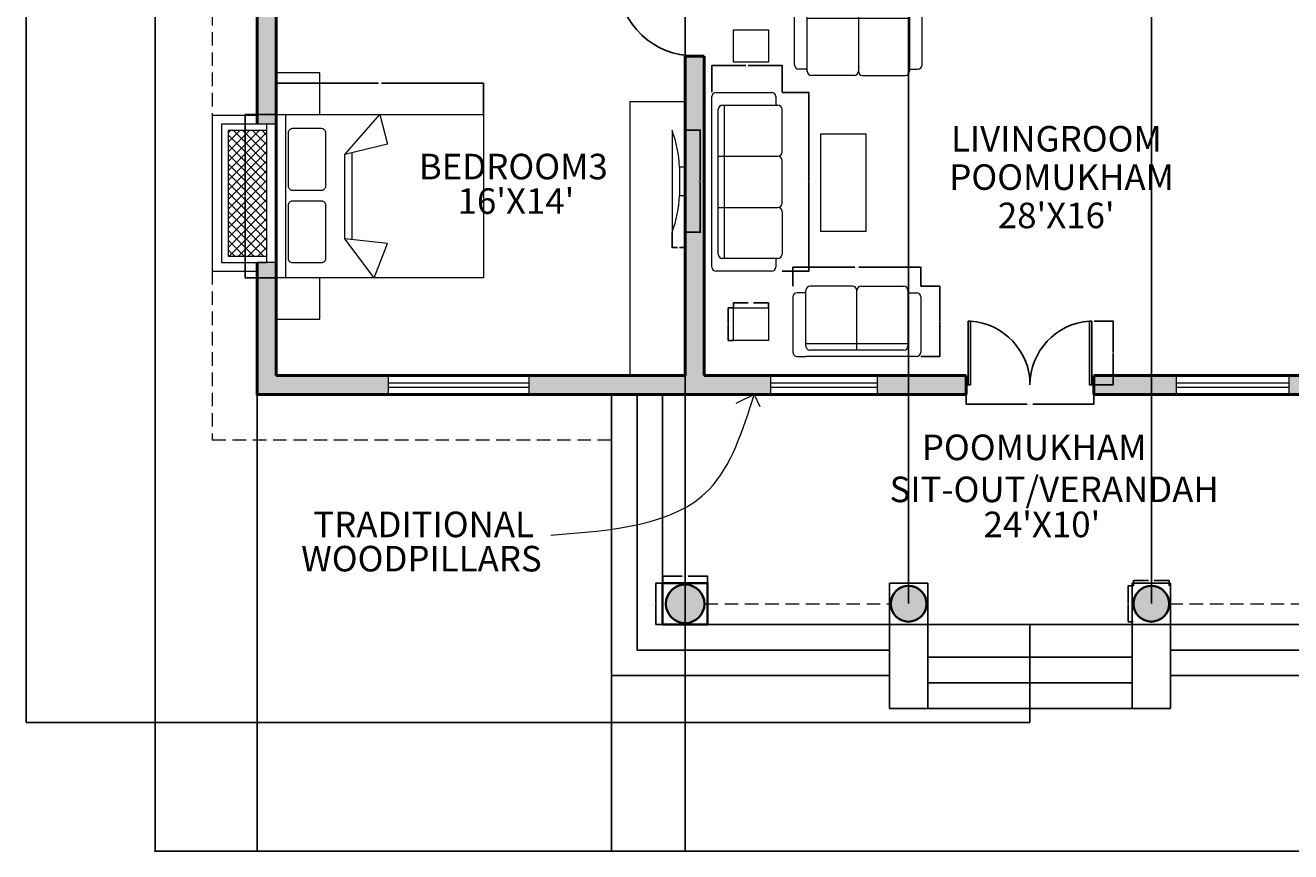
# Model space of a CAD drawing. Units: inches. Extents: x 2743 to 3669, y 1014 to 2282.
# Tile 1 of 5: x 2743 to 3337, y 1014 to 1403. Entities that reach past the tile are written whole.
import ezdxf

# ---------------------------------------------------------------- set-up
doc = ezdxf.new("R2010")
doc.units = ezdxf.units.IN
doc.linetypes.add('DASHED2', pattern=[9.525, 6.35, -3.175])
for name, color, linetype, lineweight in [('A-ANNO-DIMS', 2, 'Continuous', 18), ('A-ANNO-SYMB', 7, 'Continuous', 18), ('A-ANNO-TEXT', 4, 'Continuous', 18), ('A-AREA-IDEN', 4, 'Continuous', 18), ('A-COLS', 7, 'Continuous', 35), ('A-DOOR', 211, 'Continuous', 25), ('A-EQPM', 51, 'Continuous', 18), ('A-FLOR-CASE', 51, 'Continuous', 18), ('A-FLOR-STRS', 7, 'Continuous', 25), ('A-FURN', 111, 'Continuous', 18), ('A-GLAZ', 40, 'Continuous', 20), ('A-GLAZ-PATT', 8, 'Continuous', 13), ('A-ROOF', 7, 'Continuous', 20), ('A-ROOF-OVHD', 8, 'DASHED2', 18), ('A-WALL', 7, 'Continuous', 50)]:
    doc.layers.add(name, color=color, linetype=linetype, lineweight=lineweight)
doc.layers.add('A-COLS-PATT', color=47, linetype='Continuous', lineweight=13, true_color=0x726c55)
doc.layers.add('A-WALL-PATT', color=47, linetype='Continuous', lineweight=13, true_color=0x726c55)
doc.styles.get("Standard").update_dxf_attribs({"font": 'arial.ttf'})
doc.dimstyles.get("Standard").update_dxf_attribs({"dimtxt": 0.18, "dimasz": 0.18, "dimexe": 0.18, "dimexo": 0.0625, "dimgap": 0.09, "dimtad": 0, "dimtih": 1, "dimtoh": 1, "dimdec": 4, "dimzin": 0, "dimdsep": 46, "dimtxsty": 'Standard', "dimcen": 0.09, "dimadec": 0, "dimazin": 0, "dimtfac": 1, "dimtdec": 4, "dimtofl": 0, "dimtmove": 0, "dimatfit": 3, "dimfxl": 1, "dimtolj": 1, "dimtzin": 0, "dimarcsym": 0})

# ---------------------------------------------------------------- blocks, each defined once
blk = doc.blocks.new('DOOR-PAIR-60IN')
for p, q in [((0, 30), (1, 30)), ((1, 30), (1, 0)), ((2, 30), (1, 30)), ((2, 0), (2, 30)), ((58, 0), (58, 30)), ((58, 30), (59, 30)), ((60, 30), (59, 30)), ((59, 30), (59, 0)), ((1, 0), (2, 0)), ((59, 0), (58, 0))]:
    blk.add_line(p, q)
for centre, start, end in [((0, 29.93), 273.82241, 0.12746), ((60, 29.93), 179.99998, 266.1773)]:
    blk.add_arc(centre, 30, start, end)
blk = doc.blocks.new('DOOR-SINGLE-36IN')
for p, q in [((1, 0), (1, 36)), ((1, 36), (2, 36)), ((2, 36), (2, 0)), ((0, 0), (1, 0)), ((2, 0), (1, 0))]:
    blk.add_line(p, q)
blk.add_arc((0, 0.06), 36, 359.91152, 86.81533)
blk = doc.blocks.new('BED-DOUBLE')
for p, q in [((4.31, 76.75), (4.31, 0)), ((32.31, 57.96), (48.69, 76.75)), ((48.69, 76.75), (52.23, 62.72)), ((52.23, 62.72), (32.31, 57.96)), ((32.31, 18.34), (32.31, 57.96)), ((35.7, 17.95), (35.72, 58.78)), ((46.06, 0), (32.31, 18.34)), ((52.23, 16.05), (32.31, 18.34)), ((46.06, 0), (52.23, 16.05))]:
    blk.add_line(p, q)
blk.add_lwpolyline([(0, 76.75), (97.38, 76.75), (97.38, 0), (0, 0)], close=True)
for points in [[(7.76, 70.21), (21.16, 70.21, -0.414214), (23.16, 68.21), (23.16, 43, -0.414214), (21.16, 41), (7.76, 41, -0.414214), (5.76, 43), (5.76, 68.21, -0.414214)], [(7.76, 36.18), (21.16, 36.18, -0.414214), (23.16, 34.18), (23.16, 8.97, -0.414214), (21.16, 6.97), (7.76, 6.97, -0.414214), (5.76, 8.97), (5.76, 34.18, -0.414214)]]:
    blk.add_lwpolyline(points, format="xyb", close=True)
blk = doc.blocks.new('NIGHTSTAND')
blk.add_lwpolyline([(0, 0), (20.5, 0), (20.5, 19.45), (0, 19.45)], close=True)
blk = doc.blocks.new('TABLE-END')
blk.add_lwpolyline([(0, 15.26), (16.38, 15.26), (16.38, 0), (0, 0)], close=True)
blk = doc.blocks.new('SOFA-TWO-SEAT')
for p, q in [((5, 60), (31, 60)), ((2, 54), (28, 54)), ((3, 54), (3, 58)), ((27, 54), (27, 6)), ((33, 58), (33, 6)), ((0, 32), (0, 52)), ((30, 52), (30, 8)), ((30, 30), (2, 30)), ((2, 30), (2, 30)), ((0, 28), (0, 8)), ((28, 6), (2, 6)), ((2, 6), (2, 6)), ((3, 6), (3, 2)), ((33, 2), (33, 6)), ((5, 0), (31, 0))]:
    blk.add_line(p, q)
for centre, start, end in [((5, 58), 90, 180), ((31, 58), 0, 90), ((2, 52), 90, 180), ((28, 52), 0, 90), ((2, 32), 180, 270), ((2, 28), 90, 180), ((2, 8), 180, 270), ((28, 8), 270, 0), ((5, 2), 180, 270), ((31, 2), 270, 0)]:
    blk.add_arc(centre, 2, start, end)
blk = doc.blocks.new('SOFA-THREE-SEAT')
for p, q in [((0, 5), (0, 31)), ((2, 33), (82, 33)), ((8, 30), (76, 30)), ((30, 30), (30, 2)), ((54, 30), (54, 2)), ((84, 31), (84, 5)), ((6, 2), (6, 28)), ((6, 27), (78, 27)), ((78, 28), (78, 2)), ((6, 3), (2, 3)), ((30, 2), (30, 2)), ((54, 2), (54, 2)), ((82, 3), (78, 3)), ((28, 0), (8, 0)), ((32, 0), (52, 0)), ((56, 0), (76, 0))]:
    blk.add_line(p, q)
for centre, start, end in [((2, 31), 90, 180), ((8, 28), 90, 180), ((76, 28), 0, 90), ((82, 31), 0, 90), ((2, 5), 180, 270), ((8, 2), 180, 270), ((28, 2), 270, 0), ((32, 2), 180, 270), ((52, 2), 270, 0), ((56, 2), 180, 270), ((76, 2), 270, 0), ((82, 5), 270, 0)]:
    blk.add_arc(centre, 2, start, end)
blk = doc.blocks.new('TV-SCREEN')
for p, q in [((6.11, 0), (6.11, 47.89)), ((2.64, 30.63), (0, 30.63)), ((2.64, 17.25), (2.64, 30.63)), ((0, 17.25), (2.64, 17.25))]:
    blk.add_line(p, q)
for centre, radius, start, end in [((54.67, 29.14), 52.05, 158.88993, 178.35791), ((54.74, 18.76), 52.13, 181.66464, 201.09645)]:
    blk.add_arc(centre, radius, start, end)
blk = doc.blocks.new('POST-SITOUT-OUTER')
blk.add_lwpolyline([(0, 0), (21.09, 0), (21.09, 19.48), (0, 19.48)], close=True)
blk.add_circle((10.55, 9.74), 9.06)
blk = doc.blocks.new('POST-SITOUT-INNER')
blk.add_circle((8.4, 8.4), 8.4)
blk = doc.blocks.new('*D30')
at = {"layer": 'A-ANNO-DIMS', "color": 0, "lineweight": -2, "transparency": 16777216}
for p, q in [((2860.8, 1360.75), (2860.8, 1375.47)), ((2860.98, 1375.29), (2908.67, 1375.29)), ((2958, 1375.29), (2910.31, 1375.29)), ((2958.18, 1360.75), (2958.18, 1375.47))]:
    blk.add_line(p, q, dxfattribs=at)
at = {"layer": 'A-ANNO-DIMS', "color": 0, "transparency": 16777216}
for points in [[(2860.98, 1375.32), (2860.98, 1375.26), (2860.8, 1375.29)], [(2958, 1375.32), (2958, 1375.26), (2958.18, 1375.29)]]:
    blk.add_solid(points, dxfattribs=at)
at = {"layer": 'Defpoints', "color": 0, "transparency": 16777216}
for p in [(2958.18, 1375.29), (2860.8, 1360.68), (2958.18, 1360.68)]:
    blk.add_point(p, dxfattribs=at)
at = {"layer": 'A-ANNO-DIMS', "color": 0, "transparency": 16777216, "insert": (2909.49, 1375.29), "char_height": 0.18, "attachment_point": 5}
blk.add_mtext('\\A1;BED 97 TYP.', dxfattribs=at)
blk = doc.blocks.new('*D31')
at = {"layer": 'A-ANNO-DIMS', "color": 0, "lineweight": -2, "transparency": 16777216}
for p, q in [((2860.73, 1360.68), (2846.01, 1360.68)), ((2846.19, 1360.5), (2846.19, 1322.49)), ((2846.19, 1284.12), (2846.19, 1322.13)), ((2860.73, 1283.94), (2846.01, 1283.94))]:
    blk.add_line(p, q, dxfattribs=at)
at = {"layer": 'A-ANNO-DIMS', "color": 0, "transparency": 16777216}
for points in [[(2846.16, 1360.5), (2846.22, 1360.5), (2846.19, 1360.68)], [(2846.16, 1284.12), (2846.22, 1284.12), (2846.19, 1283.94)]]:
    blk.add_solid(points, dxfattribs=at)
at = {"layer": 'Defpoints', "color": 0, "transparency": 16777216}
for p in [(2846.19, 1360.68), (2860.8, 1360.68), (2860.8, 1283.94)]:
    blk.add_point(p, dxfattribs=at)
at = {"layer": 'A-ANNO-DIMS', "color": 0, "transparency": 16777216, "insert": (2846.19, 1322.31), "char_height": 0.18, "attachment_point": 5}
blk.add_mtext('\\A1;77 TYP.', dxfattribs=at)
blk = doc.blocks.new('*D32')
at = {"layer": 'A-ANNO-DIMS', "color": 0, "lineweight": -2, "transparency": 16777216}
for p, q in [((3184.8, 1233.53), (3184.8, 1224.41)), ((3244.8, 1233.53), (3244.8, 1224.41)), ((3184.98, 1224.59), (3213.53, 1224.59)), ((3244.62, 1224.59), (3216.06, 1224.59))]:
    blk.add_line(p, q, dxfattribs=at)
at = {"layer": 'A-ANNO-DIMS', "color": 0, "transparency": 16777216}
for points in [[(3184.98, 1224.62), (3184.98, 1224.56), (3184.8, 1224.59)], [(3244.62, 1224.62), (3244.62, 1224.56), (3244.8, 1224.59)]]:
    blk.add_solid(points, dxfattribs=at)
at = {"layer": 'Defpoints', "color": 0, "transparency": 16777216}
for p in [(3184.8, 1233.59), (3244.8, 1233.59), (3184.8, 1224.59)]:
    blk.add_point(p, dxfattribs=at)
at = {"layer": 'A-ANNO-DIMS', "color": 0, "transparency": 16777216, "insert": (3214.8, 1224.59), "char_height": 0.18, "attachment_point": 5}
blk.add_mtext('\\A1;DOOR PAIR 60 TYP.', dxfattribs=at)
blk = doc.blocks.new('*D33')
at = {"layer": 'A-ANNO-DIMS', "color": 0, "lineweight": -2, "transparency": 16777216}
for p, q in [((3244.86, 1263.59), (3253.98, 1263.59)), ((3253.8, 1263.41), (3253.8, 1248.78)), ((3253.8, 1233.77), (3253.8, 1248.41)), ((3244.86, 1233.59), (3253.98, 1233.59))]:
    blk.add_line(p, q, dxfattribs=at)
at = {"layer": 'A-ANNO-DIMS', "color": 0, "transparency": 16777216}
for points in [[(3253.83, 1263.41), (3253.77, 1263.41), (3253.8, 1263.59)], [(3253.83, 1233.77), (3253.77, 1233.77), (3253.8, 1233.59)]]:
    blk.add_solid(points, dxfattribs=at)
at = {"layer": 'Defpoints', "color": 0, "transparency": 16777216}
for p in [(3244.8, 1263.59), (3244.8, 1233.59), (3253.8, 1233.59)]:
    blk.add_point(p, dxfattribs=at)
at = {"layer": 'A-ANNO-DIMS', "color": 0, "transparency": 16777216, "insert": (3253.8, 1248.59), "char_height": 0.18, "attachment_point": 5}
blk.add_mtext('\\A1;30 TYP.', dxfattribs=at)
blk = doc.blocks.new('*D38')
at = {"layer": 'A-ANNO-DIMS', "color": 0, "lineweight": -2, "transparency": 16777216}
for p, q in [((3103.49, 1280.01), (3103.49, 1289.12)), ((3103.67, 1288.94), (3132.59, 1288.94)), ((3163.31, 1288.94), (3134.4, 1288.94)), ((3163.49, 1280.01), (3163.49, 1289.12))]:
    blk.add_line(p, q, dxfattribs=at)
at = {"layer": 'A-ANNO-DIMS', "color": 0, "transparency": 16777216}
for points in [[(3103.67, 1288.97), (3103.67, 1288.91), (3103.49, 1288.94)], [(3163.31, 1288.97), (3163.31, 1288.91), (3163.49, 1288.94)]]:
    blk.add_solid(points, dxfattribs=at)
at = {"layer": 'Defpoints', "color": 0, "transparency": 16777216}
for p in [(3163.49, 1288.94), (3103.49, 1279.94), (3163.49, 1279.94)]:
    blk.add_point(p, dxfattribs=at)
at = {"layer": 'A-ANNO-DIMS', "color": 0, "transparency": 16777216, "insert": (3133.49, 1288.94), "char_height": 0.18, "attachment_point": 5}
blk.add_mtext('\\A1;SOFA 60 TYP.', dxfattribs=at)
blk = doc.blocks.new('*D39')
at = {"layer": 'A-ANNO-DIMS', "color": 0, "lineweight": -2, "transparency": 16777216}
for p, q in [((3163.56, 1279.94), (3172.67, 1279.94)), ((3172.49, 1279.76), (3172.49, 1263.63)), ((3172.49, 1247.12), (3172.49, 1263.26)), ((3163.56, 1246.94), (3172.67, 1246.94))]:
    blk.add_line(p, q, dxfattribs=at)
at = {"layer": 'A-ANNO-DIMS', "color": 0, "transparency": 16777216}
for points in [[(3172.46, 1279.76), (3172.52, 1279.76), (3172.49, 1279.94)], [(3172.46, 1247.12), (3172.52, 1247.12), (3172.49, 1246.94)]]:
    blk.add_solid(points, dxfattribs=at)
at = {"layer": 'Defpoints', "color": 0, "transparency": 16777216}
for p in [(3163.49, 1279.94), (3163.49, 1246.94), (3172.49, 1246.94)]:
    blk.add_point(p, dxfattribs=at)
at = {"layer": 'A-ANNO-DIMS', "color": 0, "transparency": 16777216, "insert": (3172.49, 1263.44), "char_height": 0.18, "attachment_point": 5}
blk.add_mtext('\\A1;33 TYP.', dxfattribs=at)
blk = doc.blocks.new('*D46')
at = {"layer": 'A-ANNO-DIMS', "color": 0, "lineweight": -2, "transparency": 16777216}
for p, q in [((3052.86, 1353.19), (3060.16, 1353.19)), ((3059.98, 1353.01), (3059.98, 1329.42)), ((3059.98, 1305.48), (3059.98, 1329.06)), ((3052.86, 1305.3), (3060.16, 1305.3))]:
    blk.add_line(p, q, dxfattribs=at)
at = {"layer": 'A-ANNO-DIMS', "color": 0, "transparency": 16777216}
for points in [[(3059.95, 1353.01), (3060.01, 1353.01), (3059.98, 1353.19)], [(3059.95, 1305.48), (3060.01, 1305.48), (3059.98, 1305.3)]]:
    blk.add_solid(points, dxfattribs=at)
at = {"layer": 'Defpoints', "color": 0, "transparency": 16777216}
for p in [(3052.8, 1353.19), (3052.8, 1305.3), (3059.98, 1305.3)]:
    blk.add_point(p, dxfattribs=at)
at = {"layer": 'A-ANNO-DIMS', "color": 0, "transparency": 16777216, "insert": (3059.98, 1329.24), "char_height": 0.18, "attachment_point": 5}
blk.add_mtext('\\A1;SCREEN 48 TYP.', dxfattribs=at)
blk = doc.blocks.new('*D47')
at = {"layer": 'A-ANNO-DIMS', "color": 0, "lineweight": -2, "transparency": 16777216}
for p, q in [((3046.69, 1305.23), (3046.69, 1297.93)), ((3052.8, 1305.23), (3052.8, 1297.93)), ((3046.87, 1298.11), (3049.28, 1298.11)), ((3052.62, 1298.11), (3050.2, 1298.11))]:
    blk.add_line(p, q, dxfattribs=at)
at = {"layer": 'A-ANNO-DIMS', "color": 0, "transparency": 16777216}
for points in [[(3046.87, 1298.14), (3046.87, 1298.08), (3046.69, 1298.11)], [(3052.62, 1298.14), (3052.62, 1298.08), (3052.8, 1298.11)]]:
    blk.add_solid(points, dxfattribs=at)
at = {"layer": 'Defpoints', "color": 0, "transparency": 16777216}
for p in [(3046.69, 1305.3), (3052.8, 1305.3), (3046.69, 1298.11)]:
    blk.add_point(p, dxfattribs=at)
at = {"layer": 'A-ANNO-DIMS', "color": 0, "transparency": 16777216, "insert": (3049.74, 1298.11), "char_height": 0.18, "attachment_point": 5}
blk.add_mtext('\\A1;6 TYP.', dxfattribs=at)
blk = doc.blocks.new('*D54')
at = {"layer": 'A-ANNO-DIMS', "color": 0, "lineweight": -2, "transparency": 16777216}
for p, q in [((3075.58, 1269.82), (3075.58, 1272.39)), ((3075.76, 1272.21), (3082.52, 1272.21)), ((3091.79, 1272.21), (3085.03, 1272.21)), ((3091.97, 1269.82), (3091.97, 1272.39))]:
    blk.add_line(p, q, dxfattribs=at)
at = {"layer": 'A-ANNO-DIMS', "color": 0, "transparency": 16777216}
for points in [[(3075.76, 1272.24), (3075.76, 1272.18), (3075.58, 1272.21)], [(3091.79, 1272.24), (3091.79, 1272.18), (3091.97, 1272.21)]]:
    blk.add_solid(points, dxfattribs=at)
at = {"layer": 'Defpoints', "color": 0, "transparency": 16777216}
for p in [(3091.97, 1272.21), (3075.58, 1269.76), (3091.97, 1269.76)]:
    blk.add_point(p, dxfattribs=at)
at = {"layer": 'A-ANNO-DIMS', "color": 0, "transparency": 16777216, "insert": (3083.77, 1272.21), "char_height": 0.18, "attachment_point": 5}
blk.add_mtext('\\A1;END TABLE 16 TYP.', dxfattribs=at)
blk = doc.blocks.new('*D55')
at = {"layer": 'A-ANNO-DIMS', "color": 0, "lineweight": -2, "transparency": 16777216}
for p, q in [((3075.52, 1269.76), (3072.94, 1269.76)), ((3073.12, 1269.58), (3073.12, 1262.31)), ((3073.12, 1254.67), (3073.12, 1261.94)), ((3075.52, 1254.49), (3072.94, 1254.49))]:
    blk.add_line(p, q, dxfattribs=at)
at = {"layer": 'A-ANNO-DIMS', "color": 0, "transparency": 16777216}
for points in [[(3073.09, 1269.58), (3073.15, 1269.58), (3073.12, 1269.76)], [(3073.09, 1254.67), (3073.15, 1254.67), (3073.12, 1254.49)]]:
    blk.add_solid(points, dxfattribs=at)
at = {"layer": 'Defpoints', "color": 0, "transparency": 16777216}
for p in [(3073.12, 1269.76), (3075.58, 1269.76), (3075.58, 1254.49)]:
    blk.add_point(p, dxfattribs=at)
at = {"layer": 'A-ANNO-DIMS', "color": 0, "transparency": 16777216, "insert": (3073.12, 1262.12), "char_height": 0.18, "attachment_point": 5}
blk.add_mtext('\\A1;15 TYP.', dxfattribs=at)
blk = doc.blocks.new('*D56')
at = {"layer": 'A-ANNO-DIMS', "color": 0, "lineweight": -2, "transparency": 16777216}
for p, q in [((3098.44, 1371), (3111.16, 1371)), ((3110.98, 1370.82), (3110.98, 1329.18)), ((3110.98, 1287.18), (3110.98, 1328.82)), ((3098.44, 1287), (3111.16, 1287))]:
    blk.add_line(p, q, dxfattribs=at)
at = {"layer": 'A-ANNO-DIMS', "color": 0, "transparency": 16777216}
for points in [[(3110.95, 1370.82), (3111.01, 1370.82), (3110.98, 1371)], [(3110.95, 1287.18), (3111.01, 1287.18), (3110.98, 1287)]]:
    blk.add_solid(points, dxfattribs=at)
at = {"layer": 'Defpoints', "color": 0, "transparency": 16777216}
for p in [(3098.38, 1371), (3110.98, 1371), (3098.38, 1287)]:
    blk.add_point(p, dxfattribs=at)
at = {"layer": 'A-ANNO-DIMS', "color": 0, "transparency": 16777216, "insert": (3110.98, 1329), "char_height": 0.18, "attachment_point": 5}
blk.add_mtext('\\A1;SOFA 84 TYP.', dxfattribs=at)
blk = doc.blocks.new('*D57')
at = {"layer": 'A-ANNO-DIMS', "color": 0, "lineweight": -2, "transparency": 16777216}
for p, q in [((3065.38, 1371.06), (3065.38, 1383.78)), ((3065.56, 1383.6), (3081.35, 1383.6)), ((3098.2, 1383.6), (3082.41, 1383.6)), ((3098.38, 1371.06), (3098.38, 1383.78))]:
    blk.add_line(p, q, dxfattribs=at)
at = {"layer": 'A-ANNO-DIMS', "color": 0, "transparency": 16777216}
for points in [[(3065.56, 1383.63), (3065.56, 1383.57), (3065.38, 1383.6)], [(3098.2, 1383.63), (3098.2, 1383.57), (3098.38, 1383.6)]]:
    blk.add_solid(points, dxfattribs=at)
at = {"layer": 'Defpoints', "color": 0, "transparency": 16777216}
for p in [(3065.38, 1383.6), (3065.38, 1371), (3098.38, 1371)]:
    blk.add_point(p, dxfattribs=at)
at = {"layer": 'A-ANNO-DIMS', "color": 0, "transparency": 16777216, "insert": (3081.88, 1383.6), "char_height": 0.18, "attachment_point": 5}
blk.add_mtext('\\A1;33 TYP.', dxfattribs=at)
blk = doc.blocks.new('*D58')
at = {"layer": 'A-ANNO-DIMS', "color": 0, "lineweight": -2, "transparency": 16777216}
for p, q in [((3042.3, 1140.64), (3042.3, 1143.92)), ((3042.48, 1143.74), (3051.46, 1143.74)), ((3063.21, 1143.74), (3054.22, 1143.74)), ((3063.39, 1140.64), (3063.39, 1143.92))]:
    blk.add_line(p, q, dxfattribs=at)
at = {"layer": 'A-ANNO-DIMS', "color": 0, "transparency": 16777216}
for points in [[(3042.48, 1143.77), (3042.48, 1143.71), (3042.3, 1143.74)], [(3063.21, 1143.77), (3063.21, 1143.71), (3063.39, 1143.74)]]:
    blk.add_solid(points, dxfattribs=at)
at = {"layer": 'Defpoints', "color": 0, "transparency": 16777216}
for p in [(3063.39, 1143.74), (3042.3, 1140.58), (3063.39, 1140.58)]:
    blk.add_point(p, dxfattribs=at)
at = {"layer": 'A-ANNO-DIMS', "color": 0, "transparency": 16777216, "insert": (3052.84, 1143.74), "char_height": 0.18, "attachment_point": 5}
blk.add_mtext('\\A1;OUTER POST 21 TYP.', dxfattribs=at)
blk = doc.blocks.new('*D59')
at = {"layer": 'A-ANNO-DIMS', "color": 0, "lineweight": -2, "transparency": 16777216}
for p, q in [((3042.23, 1140.58), (3038.95, 1140.58)), ((3039.13, 1140.4), (3039.13, 1131.02)), ((3039.13, 1121.27), (3039.13, 1130.65)), ((3042.23, 1121.09), (3038.95, 1121.09))]:
    blk.add_line(p, q, dxfattribs=at)
at = {"layer": 'A-ANNO-DIMS', "color": 0, "transparency": 16777216}
for points in [[(3039.1, 1140.4), (3039.16, 1140.4), (3039.13, 1140.58)], [(3039.1, 1121.27), (3039.16, 1121.27), (3039.13, 1121.09)]]:
    blk.add_solid(points, dxfattribs=at)
at = {"layer": 'Defpoints', "color": 0, "transparency": 16777216}
for p in [(3039.13, 1140.58), (3042.3, 1140.58), (3042.3, 1121.09)]:
    blk.add_point(p, dxfattribs=at)
at = {"layer": 'A-ANNO-DIMS', "color": 0, "transparency": 16777216, "insert": (3039.13, 1130.83), "char_height": 0.18, "attachment_point": 5}
blk.add_mtext('\\A1;19 TYP.', dxfattribs=at)
blk = doc.blocks.new('*D60')
at = {"layer": 'A-ANNO-DIMS', "color": 0, "lineweight": -2, "transparency": 16777216}
for p, q in [((3263.39, 1139.3), (3263.39, 1141.94)), ((3263.57, 1141.76), (3270.47, 1141.76)), ((3280.02, 1141.76), (3273.12, 1141.76)), ((3280.2, 1139.3), (3280.2, 1141.94))]:
    blk.add_line(p, q, dxfattribs=at)
at = {"layer": 'A-ANNO-DIMS', "color": 0, "transparency": 16777216}
for points in [[(3263.57, 1141.79), (3263.57, 1141.73), (3263.39, 1141.76)], [(3280.02, 1141.79), (3280.02, 1141.73), (3280.2, 1141.76)]]:
    blk.add_solid(points, dxfattribs=at)
at = {"layer": 'Defpoints', "color": 0, "transparency": 16777216}
for p in [(3280.2, 1141.76), (3263.39, 1139.24), (3280.2, 1139.24)]:
    blk.add_point(p, dxfattribs=at)
at = {"layer": 'A-ANNO-DIMS', "color": 0, "transparency": 16777216, "insert": (3271.8, 1141.76), "char_height": 0.18, "attachment_point": 5}
blk.add_mtext('\\A1;INNER POST 17 TYP.', dxfattribs=at)
blk = doc.blocks.new('*D61')
at = {"layer": 'A-ANNO-DIMS', "color": 0, "lineweight": -2, "transparency": 16777216}
for p, q in [((3263.33, 1139.24), (3260.69, 1139.24)), ((3260.87, 1139.06), (3260.87, 1131.02)), ((3260.87, 1122.61), (3260.87, 1130.65)), ((3263.33, 1122.43), (3260.69, 1122.43))]:
    blk.add_line(p, q, dxfattribs=at)
at = {"layer": 'A-ANNO-DIMS', "color": 0, "transparency": 16777216}
for points in [[(3260.84, 1139.06), (3260.9, 1139.06), (3260.87, 1139.24)], [(3260.84, 1122.61), (3260.9, 1122.61), (3260.87, 1122.43)]]:
    blk.add_solid(points, dxfattribs=at)
at = {"layer": 'Defpoints', "color": 0, "transparency": 16777216}
for p in [(3260.87, 1139.24), (3263.39, 1139.24), (3263.39, 1122.43)]:
    blk.add_point(p, dxfattribs=at)
at = {"layer": 'A-ANNO-DIMS', "color": 0, "transparency": 16777216, "insert": (3260.87, 1130.83), "char_height": 0.18, "attachment_point": 5}
blk.add_mtext('\\A1;17 TYP.', dxfattribs=at)
blk = doc.blocks.new('*D62')
at = {"layer": 'A-ANNO-DIMS', "color": 0, "lineweight": -2, "transparency": 16777216}
for p, q in [((3608.38, 1899.55), (3608.38, 1014.41)), ((2803.91, 1765.52), (2803.91, 1014.41)), ((2804.09, 1014.59), (3205.75, 1014.59)), ((3608.2, 1014.59), (3206.54, 1014.59))]:
    blk.add_line(p, q, dxfattribs=at)
at = {"layer": 'A-ANNO-DIMS', "color": 0, "transparency": 16777216}
for points in [[(2804.09, 1014.62), (2804.09, 1014.56), (2803.91, 1014.59)], [(3608.2, 1014.62), (3608.2, 1014.56), (3608.38, 1014.59)]]:
    blk.add_solid(points, dxfattribs=at)
at = {"layer": 'Defpoints', "color": 0, "transparency": 16777216}
for p in [(3608.38, 1899.61), (2803.91, 1765.58), (3608.38, 1014.59)]:
    blk.add_point(p, dxfattribs=at)
at = {"layer": 'A-ANNO-DIMS', "color": 0, "transparency": 16777216, "insert": (3206.15, 1014.59), "char_height": 0.18, "attachment_point": 5}
blk.add_mtext('\\A1;804.5', dxfattribs=at)
blk = doc.blocks.new('*D63')
at = {"layer": 'A-ANNO-DIMS', "color": 0, "lineweight": -2, "transparency": 16777216}
for p, q in [((3001.57, 2220.87), (2743.18, 2220.87)), ((2743.36, 2220.69), (2743.36, 1648.19)), ((2743.36, 1075.32), (2743.36, 1647.82)), ((3214.73, 1075.14), (2743.18, 1075.14))]:
    blk.add_line(p, q, dxfattribs=at)
at = {"layer": 'A-ANNO-DIMS', "color": 0, "transparency": 16777216}
for points in [[(2743.33, 2220.69), (2743.39, 2220.69), (2743.36, 2220.87)], [(2743.33, 1075.32), (2743.39, 1075.32), (2743.36, 1075.14)]]:
    blk.add_solid(points, dxfattribs=at)
at = {"layer": 'Defpoints', "color": 0, "transparency": 16777216}
for p in [(2743.36, 2220.87), (3001.63, 2220.87), (3214.8, 1075.14)]:
    blk.add_point(p, dxfattribs=at)
at = {"layer": 'A-ANNO-DIMS', "color": 0, "transparency": 16777216, "insert": (2743.36, 1648.01), "char_height": 0.18, "attachment_point": 5}
blk.add_mtext('\\A1;1145.7', dxfattribs=at)
blk = doc.blocks.new('*D73')
at = {"layer": 'A-ANNO-DIMS', "color": 0, "lineweight": -2, "transparency": 16777216}
for p, q in [((3052.8, 1238.03), (3052.8, 1014.41)), ((2851.8, 1229.03), (2851.8, 1014.41)), ((2851.98, 1014.59), (2952.02, 1014.59)), ((3052.62, 1014.59), (2952.57, 1014.59))]:
    blk.add_line(p, q, dxfattribs=at)
at = {"layer": 'A-ANNO-DIMS', "color": 0, "transparency": 16777216}
for points in [[(2851.98, 1014.62), (2851.98, 1014.56), (2851.8, 1014.59)], [(3052.62, 1014.62), (3052.62, 1014.56), (3052.8, 1014.59)]]:
    blk.add_solid(points, dxfattribs=at)
at = {"layer": 'Defpoints', "color": 0, "transparency": 16777216}
for p in [(3052.8, 1238.09), (2851.8, 1229.09), (3052.8, 1014.59)]:
    blk.add_point(p, dxfattribs=at)
at = {"layer": 'A-ANNO-DIMS', "color": 0, "transparency": 16777216, "insert": (2952.3, 1014.59), "char_height": 0.18, "attachment_point": 5}
blk.add_mtext('\\A1;201', dxfattribs=at)
blk = doc.blocks.new('*D74')
at = {"layer": 'A-ANNO-DIMS', "color": 0, "lineweight": -2, "transparency": 16777216}
for p, q in [((3052.8, 1238.03), (3052.8, 1014.41)), ((3376.8, 1238.03), (3376.8, 1014.41)), ((3052.98, 1014.59), (3214.51, 1014.59)), ((3376.62, 1014.59), (3215.08, 1014.59))]:
    blk.add_line(p, q, dxfattribs=at)
at = {"layer": 'A-ANNO-DIMS', "color": 0, "transparency": 16777216}
for points in [[(3052.98, 1014.62), (3052.98, 1014.56), (3052.8, 1014.59)], [(3376.62, 1014.62), (3376.62, 1014.56), (3376.8, 1014.59)]]:
    blk.add_solid(points, dxfattribs=at)
at = {"layer": 'Defpoints', "color": 0, "transparency": 16777216}
for p in [(3052.8, 1238.09), (3376.8, 1238.09), (3376.8, 1014.59)]:
    blk.add_point(p, dxfattribs=at)
at = {"layer": 'A-ANNO-DIMS', "color": 0, "transparency": 16777216, "insert": (3214.8, 1014.59), "char_height": 0.18, "attachment_point": 5}
blk.add_mtext('\\A1;324', dxfattribs=at)
blk = doc.blocks.new('*D75')
at = {"layer": 'A-ANNO-DIMS', "color": 0, "lineweight": -2, "transparency": 16777216}
for p, q in [((3018.3, 1097.03), (3018.3, 1014.41)), ((3411.3, 1097.03), (3411.3, 1014.41)), ((3018.48, 1014.59), (3214.51, 1014.59)), ((3411.12, 1014.59), (3215.09, 1014.59))]:
    blk.add_line(p, q, dxfattribs=at)
at = {"layer": 'A-ANNO-DIMS', "color": 0, "transparency": 16777216}
for points in [[(3018.48, 1014.62), (3018.48, 1014.56), (3018.3, 1014.59)], [(3411.12, 1014.62), (3411.12, 1014.56), (3411.3, 1014.59)]]:
    blk.add_solid(points, dxfattribs=at)
at = {"layer": 'Defpoints', "color": 0, "transparency": 16777216}
for p in [(3018.3, 1097.09), (3411.3, 1097.09), (3411.3, 1014.59)]:
    blk.add_point(p, dxfattribs=at)
at = {"layer": 'A-ANNO-DIMS', "color": 0, "transparency": 16777216, "insert": (3214.8, 1014.59), "char_height": 0.18, "attachment_point": 5}
blk.add_mtext('\\A1;393', dxfattribs=at)
blk = doc.blocks.new('*D76')
at = {"layer": 'A-ANNO-DIMS', "color": 0, "lineweight": -2, "transparency": 16777216}
for p, q in [((3052.84, 1130.9), (3052.84, 2281.6)), ((3053.02, 2281.42), (3104.86, 2281.42)), ((3157.62, 2281.42), (3105.77, 2281.42)), ((3157.8, 1130.9), (3157.8, 2281.6))]:
    blk.add_line(p, q, dxfattribs=at)
at = {"layer": 'A-ANNO-DIMS', "color": 0, "transparency": 16777216}
for points in [[(3053.02, 2281.45), (3053.02, 2281.39), (3052.84, 2281.42)], [(3157.62, 2281.45), (3157.62, 2281.39), (3157.8, 2281.42)]]:
    blk.add_solid(points, dxfattribs=at)
at = {"layer": 'Defpoints', "color": 0, "transparency": 16777216}
for p in [(3157.8, 2281.42), (3052.84, 1130.83), (3157.8, 1130.83)]:
    blk.add_point(p, dxfattribs=at)
at = {"layer": 'A-ANNO-DIMS', "color": 0, "transparency": 16777216, "insert": (3105.32, 2281.42), "char_height": 0.18, "attachment_point": 5}
blk.add_mtext('\\A1;104.95', dxfattribs=at)
blk = doc.blocks.new('*D77')
at = {"layer": 'A-ANNO-DIMS', "color": 0, "lineweight": -2, "transparency": 16777216}
for p, q in [((3157.8, 1130.9), (3157.8, 2281.6)), ((3157.98, 2281.42), (3214.52, 2281.42)), ((3271.62, 2281.42), (3215.08, 2281.42)), ((3271.8, 1130.9), (3271.8, 2281.6))]:
    blk.add_line(p, q, dxfattribs=at)
at = {"layer": 'A-ANNO-DIMS', "color": 0, "transparency": 16777216}
for points in [[(3157.98, 2281.45), (3157.98, 2281.39), (3157.8, 2281.42)], [(3271.62, 2281.45), (3271.62, 2281.39), (3271.8, 2281.42)]]:
    blk.add_solid(points, dxfattribs=at)
at = {"layer": 'Defpoints', "color": 0, "transparency": 16777216}
for p in [(3271.8, 2281.42), (3157.8, 1130.83), (3271.8, 1130.83)]:
    blk.add_point(p, dxfattribs=at)
at = {"layer": 'A-ANNO-DIMS', "color": 0, "transparency": 16777216, "insert": (3214.8, 2281.42), "char_height": 0.18, "attachment_point": 5}
blk.add_mtext('\\A1;114', dxfattribs=at)
blk = doc.blocks.new('*D78')
at = {"layer": 'A-ANNO-DIMS', "color": 0, "lineweight": -2, "transparency": 16777216}
for p, q in [((3271.8, 1130.9), (3271.8, 2281.6)), ((3271.98, 2281.42), (3323.82, 2281.42)), ((3376.57, 2281.42), (3324.73, 2281.42)), ((3376.75, 1130.9), (3376.75, 2281.6))]:
    blk.add_line(p, q, dxfattribs=at)
at = {"layer": 'A-ANNO-DIMS', "color": 0, "transparency": 16777216}
for points in [[(3271.98, 2281.45), (3271.98, 2281.39), (3271.8, 2281.42)], [(3376.57, 2281.45), (3376.57, 2281.39), (3376.75, 2281.42)]]:
    blk.add_solid(points, dxfattribs=at)
at = {"layer": 'Defpoints', "color": 0, "transparency": 16777216}
for p in [(3376.75, 2281.42), (3271.8, 1130.83), (3376.75, 1130.83)]:
    blk.add_point(p, dxfattribs=at)
at = {"layer": 'A-ANNO-DIMS', "color": 0, "transparency": 16777216, "insert": (3324.27, 2281.42), "char_height": 0.18, "attachment_point": 5}
blk.add_mtext('\\A1;104.95', dxfattribs=at)

msp = doc.modelspace()

# ---------------------------------------------------------------- hatches: boundary and pattern name
at = {"layer": 'A-COLS-PATT'}
h = msp.add_hatch(color=256, dxfattribs=at)
h.dxf.hatch_style = 1
h.paths.add_polyline_path([(3061.905, 1130.835, 1), (3043.779, 1130.835, 1)])
h = msp.add_hatch(color=256, dxfattribs=at)
h.dxf.hatch_style = 1
h.paths.add_polyline_path([(3166.201, 1130.835, 1), (3149.392, 1130.835, 1)])
h = msp.add_hatch(color=256, dxfattribs=at)
h.dxf.hatch_style = 1
h.paths.add_polyline_path([(3280.201, 1130.835, 1), (3263.392, 1130.835, 1)])
at = {"layer": 'A-GLAZ-PATT'}
h = msp.add_hatch(dxfattribs=at)
h.set_pattern_fill('ANSI37', color=256)
h.paths.add_polyline_path([(2856.296, 1353.075), (2838.296, 1353.075), (2838.296, 1294.075), (2856.296, 1294.075)])
at = {"layer": 'A-WALL-PATT'}
h = msp.add_hatch(color=256, dxfattribs=at)
h.dxf.hatch_style = 1
h.paths.add_polyline_path([(2851.796, 1356.075), (2856.296, 1356.075), (2860.796, 1356.075), (2860.796, 1360.685), (2860.796, 1380.133), (2860.796, 1430.094), (2955.206, 1430.094), (2962.796, 1430.094), (2962.796, 1445.094), (2956.796, 1445.094), (2956.796, 1439.094), (2860.796, 1439.094), (2860.796, 1443.244), (2860.771, 1443.244), (2860.771, 1456.626), (2860.775, 1465.516), (2851.796, 1465.516)])
h = msp.add_hatch(color=256, dxfattribs=at)
h.dxf.hatch_style = 1
h.paths.add_polyline_path([(3092.989, 1229.094), (3092.989, 1238.094), (3061.796, 1238.094), (3061.796, 1388.094), (3052.796, 1388.094), (3052.796, 1238.094), (3027.084, 1238.094), (2979.416, 1238.094), (2979.416, 1229.094)])
h = msp.add_hatch(color=256, dxfattribs=at)
h.dxf.hatch_style = 1
h.paths.add_polyline_path([(3336.421, 1238.094), (3336.421, 1229.094), (3442.044, 1229.094), (3442.044, 1238.094), (3376.796, 1238.094), (3376.796, 1366.758), (3376.796, 1388.094), (3367.796, 1388.094), (3367.796, 1238.094)])
h = msp.add_hatch(color=256, dxfattribs=at)
h.dxf.hatch_style = 1
h.paths.add_polyline_path([(2851.796, 1229.094), (2913.416, 1229.094), (2913.416, 1238.094), (2860.796, 1238.094), (2860.796, 1291.05), (2851.796, 1291.05)])
h = msp.add_hatch(color=256, dxfattribs=at)
h.dxf.hatch_style = 1
h.paths.add_polyline_path([(3184.796, 1229.094), (3184.796, 1238.094), (3142.989, 1238.094), (3142.989, 1229.094)])
h = msp.add_hatch(color=256, dxfattribs=at)
h.dxf.hatch_style = 1
h.paths.add_polyline_path([(3283.421, 1229.094), (3283.421, 1238.094), (3244.796, 1238.094), (3244.796, 1229.094)])

# ---------------------------------------------------------------- linework, layer by layer
at = {"layer": 'A-ANNO-SYMB'}
for q in [(3076.583, 1224.854), (3088, 1223.554)]:
    msp.add_line((3085.308, 1229.094), q, dxfattribs=at)
msp.add_open_spline([(2989.754, 1163.094), (3018.705, 1165.303), (3066.146, 1168.922), (3079.934, 1212.219), (3085.308, 1229.094)], degree=3, knots=[0, 0, 0, 0, 77.340013, 126.7353841, 126.7353841, 126.7353841, 126.7353841], dxfattribs=at)
at = {"layer": 'A-FLOR-CASE'}
msp.add_lwpolyline([(3052.796, 1238.094), (3027.084, 1238.094), (3027.084, 1366.758), (3052.796, 1366.758)], close=True, dxfattribs=at)
at = {"layer": 'A-FLOR-STRS'}
for p, q in [((3018.296, 1229.094), (3018.296, 1097.094)), ((3030.296, 1229.094), (3030.296, 1109.094)), ((3042.296, 1229.094), (3042.296, 1121.094)), ((3166.796, 1140.575), (3148.796, 1140.575)), ((3148.796, 1140.575), (3148.796, 1097.094)), ((3166.796, 1121.094), (3166.796, 1140.575)), ((3262.796, 1121.094), (3262.796, 1140.575)), ((3262.796, 1140.575), (3280.796, 1140.575)), ((3280.796, 1140.575), (3280.796, 1097.094)), ((3042.296, 1121.094), (3387.296, 1121.094)), ((3166.796, 1097.094), (3166.796, 1121.094)), ((3214.796, 1097.094), (3214.796, 1121.094)), ((3262.796, 1097.094), (3262.796, 1121.094)), ((3030.296, 1109.094), (3148.796, 1109.094)), ((3166.796, 1105.732), (3262.796, 1105.732)), ((3280.796, 1109.094), (3399.296, 1109.094)), ((3018.296, 1097.094), (3148.796, 1097.094)), ((3148.796, 1097.094), (3148.796, 1081.732)), ((3166.796, 1081.732), (3166.796, 1097.094)), ((3166.796, 1093.732), (3262.796, 1093.732)), ((3214.796, 1097.094), (3214.796, 1075.139)), ((3262.796, 1081.732), (3262.796, 1097.094)), ((3280.796, 1097.094), (3411.296, 1097.094)), ((3280.796, 1097.094), (3280.796, 1081.732)), ((3148.796, 1081.732), (3166.796, 1081.732)), ((3166.796, 1081.732), (3262.796, 1081.732)), ((3280.796, 1081.732), (3262.796, 1081.732))]:
    msp.add_line(p, q, dxfattribs=at)
at = {"layer": 'A-FURN'}
msp.add_lwpolyline([(3116.55, 1351.591), (3137.736, 1351.591), (3137.736, 1305.728), (3116.55, 1305.728)], close=True, dxfattribs=at)
at = {"layer": 'A-GLAZ'}
for p, q in [((2856.296, 1356.075), (2835.062, 1356.075)), ((2835.062, 1356.075), (2835.062, 1291.05)), ((2860.796, 1356.075), (2851.796, 1356.075)), ((2856.296, 1356.075), (2856.296, 1291.05)), ((2856.296, 1356.075), (2856.296, 1353.075)), ((2856.296, 1353.075), (2838.296, 1353.075)), ((2838.296, 1353.075), (2838.296, 1294.075)), ((2835.062, 1291.05), (2856.296, 1291.05)), ((2838.296, 1294.075), (2856.296, 1294.075)), ((2860.796, 1291.05), (2851.796, 1291.05)), ((2913.416, 1238.094), (2913.416, 1229.094)), ((2979.416, 1238.094), (2979.416, 1229.094)), ((3092.989, 1238.094), (3092.989, 1229.094)), ((3142.989, 1238.094), (3142.989, 1229.094)), ((3283.421, 1238.094), (3283.421, 1229.094)), ((3336.421, 1238.094), (3336.421, 1229.094)), ((2913.416, 1234.594), (2979.416, 1234.594)), ((2913.416, 1232.594), (2979.416, 1232.594)), ((3092.989, 1234.594), (3142.989, 1234.594)), ((3092.989, 1232.594), (3142.989, 1232.594)), ((3283.421, 1234.594), (3336.421, 1234.594)), ((3283.421, 1232.594), (3336.421, 1232.594))]:
    msp.add_line(p, q, dxfattribs=at)
at = {"layer": 'A-ROOF'}
for p, q in [((2851.796, 1360.075), (2830.796, 1360.075)), ((2830.796, 1360.075), (2830.796, 1287.075)), ((2851.796, 1356.075), (2851.796, 1360.075)), ((2830.796, 1287.075), (2851.796, 1287.075))]:
    msp.add_line(p, q, dxfattribs=at)
at = {"layer": 'A-ROOF-OVHD'}
for p, q in [((2830.796, 1523.146), (2830.796, 1360.075)), ((2830.796, 1287.075), (2830.796, 1207.768)), ((3052.842, 1139.898), (3052.842, 1229.094)), ((2830.796, 1207.768), (3018.296, 1207.768)), ((3061.905, 1130.835), (3149.392, 1130.835)), ((3280.201, 1130.835), (3367.688, 1130.835))]:
    msp.add_line(p, q, dxfattribs=at)
at = {"layer": 'A-WALL'}
for p, q in [((2860.796, 1238.094), (2860.796, 1430.094)), ((3052.796, 1238.094), (3052.796, 1388.094)), ((3052.796, 1388.094), (3061.796, 1388.094)), ((3061.796, 1238.094), (3061.796, 1388.094)), ((3052.796, 1238.094), (2860.796, 1238.094)), ((3184.796, 1238.094), (3061.796, 1238.094)), ((3184.796, 1238.094), (3184.796, 1229.094)), ((3367.796, 1238.094), (3244.796, 1238.094)), ((3244.796, 1238.094), (3244.796, 1229.094))]:
    msp.add_line(p, q, dxfattribs=at)
for points in [[(2851.796, 1356.075), (2851.796, 1715.094)], [(3577.796, 1307.044), (3577.796, 1229.094), (3244.796, 1229.094)], [(3184.796, 1229.094), (2851.796, 1229.094), (2851.796, 1291.05)]]:
    msp.add_lwpolyline(points, dxfattribs=at)

# ---------------------------------------------------------------- block references
at = {"layer": 'A-COLS'}
for name, p in [('POST-SITOUT-OUTER', (3042.296, 1121.094)), ('POST-SITOUT-INNER', (3149.392, 1122.431)), ('POST-SITOUT-INNER', (3263.392, 1122.431))]:
    msp.add_blockref(name, p, dxfattribs=at)
at = {"layer": 'A-DOOR', "extrusion": (0, 0, -1), "zscale": -1, "rotation": 270.0000000000017}
msp.add_blockref('DOOR-SINGLE-36IN', (-3057.297, 1424.095), dxfattribs=at)
at = {"layer": 'A-DOOR', "rotation": 180.0036176401362}
msp.add_blockref('DOOR-PAIR-60IN', (3244.796, 1263.594), dxfattribs=at)
at = {"layer": 'A-EQPM', "rotation": 180}
msp.add_blockref('TV-SCREEN', (3052.797, 1353.186), dxfattribs=at)
at = {"layer": 'A-FURN'}
for name, p, rotation in [('SOFA-TWO-SEAT', (3164.19, 1378.923), 90.00000000000146), ('SOFA-THREE-SEAT', (3098.378, 1287.001), 89.99999999999872), ('SOFA-TWO-SEAT', (3103.494, 1279.944), 270.0000000000048)]:
    msp.add_blockref(name, p, dxfattribs=dict(at, rotation=rotation))
for name, p in [('TABLE-END', (3075.582, 1385.165)), ('NIGHTSTAND', (2860.796, 1360.685)), ('BED-DOUBLE', (2860.796, 1283.936)), ('NIGHTSTAND', (2860.796, 1264.488)), ('TABLE-END', (3075.582, 1254.491))]:
    msp.add_blockref(name, p, dxfattribs=at)

# ---------------------------------------------------------------- texts
at = {"layer": 'A-ANNO-TEXT'}
for tag, p in [('TRADITIONAL', (2878.214, 1162.114)), ('WOODPILLARS', (2872.528, 1146.027))]:
    msp.add_attdef(tag, p, '', height=12, dxfattribs=at)
at = {"layer": 'A-AREA-IDEN'}
for tag, p in [('LIVINGROOM', (3177.7, 1343.223)), ('BEDROOM3', (2927.789, 1330.171)), ('POOMUKHAM', (3176.899, 1325.225)), ("16'X14'", (2945.999, 1313.971)), ("28'X16'", (3199.716, 1307.228)), ('POOMUKHAM', (3164.017, 1198.302)), ('SIT-OUT/VERANDAH', (3148.871, 1178.563)), ("24'X10'", (3192.993, 1162.114))]:
    msp.add_attdef(tag, p, '', height=12, dxfattribs=at)

# ---------------------------------------------------------------- dimensions: what is measured, and where the dimension line sits
at = {"layer": 'A-ANNO-DIMS'}
for base, p1, p2, override, picture, middle in [((3157.796, 2281.421), (3052.842, 1130.835), (3157.796, 1130.835), {"dimdec": 2, "dimlfac": 1, "dimrnd": 0, "dimzin": 0, "dimdsep": 46, "dimlunit": 2}, '*D76', (3105.319, 2281.421)), ((3271.796, 2281.421), (3157.796, 1130.835), (3271.796, 1130.835), {"dimdec": 0, "dimlfac": 1, "dimrnd": 0, "dimzin": 0, "dimdsep": 46, "dimlunit": 2}, '*D77', (3214.796, 2281.421)), ((3376.7513, 2281.4212), (3271.7965, 1130.8347), (3376.7513, 1130.8347), {"dimdec": 2, "dimlfac": 1, "dimrnd": 0, "dimzin": 0, "dimdsep": 46, "dimlunit": 2}, '*D78', (3324.2739, 2281.4212)), ((3608.383, 1014.589), (2803.91, 1765.581), (3608.383, 1899.608), {"dimdec": 1, "dimlfac": 1, "dimrnd": 0, "dimzin": 0, "dimdsep": 46, "dimlunit": 2}, '*D62', (3206.146, 1014.589)), ((3052.796, 1014.589), (2851.796, 1229.094), (3052.796, 1238.094), {"dimdec": 0, "dimlfac": 1, "dimrnd": 0, "dimzin": 0, "dimdsep": 46, "dimlunit": 2}, '*D73', (2952.296, 1014.589)), ((3376.796, 1014.589), (3052.796, 1238.094), (3376.796, 1238.094), {"dimdec": 0, "dimlfac": 1, "dimrnd": 0, "dimzin": 0, "dimdsep": 46, "dimlunit": 2}, '*D74', (3214.796, 1014.589)), ((3411.296, 1014.589), (3018.296, 1097.094), (3411.296, 1097.094), {"dimdec": 0, "dimlfac": 1, "dimrnd": 0, "dimzin": 0, "dimdsep": 46, "dimlunit": 2}, '*D75', (3214.796, 1014.589))]:
    dim = msp.add_linear_dim(base=base, p1=p1, p2=p2, dimstyle='Standard', override=override, dxfattribs=at)
    dim.commit()
    dim.dimension.update_dxf_attribs({"geometry": picture, "text_midpoint": middle})
dim = msp.add_linear_dim(base=(2743.36, 2220.871), p1=(3214.796, 1075.139), p2=(3001.629, 2220.871), angle=90, dimstyle='Standard', override={"dimdec": 1, "dimlfac": 1, "dimrnd": 0, "dimzin": 0, "dimdsep": 46, "dimlunit": 2}, dxfattribs=at)
dim.commit()
dim.dimension.update_dxf_attribs({"geometry": '*D63', "text_midpoint": (2743.36, 1648.005)})
for base, p1, p2, angle, text, picture, middle in [((3065.378, 1383.601), (3098.378, 1371.001), (3065.378, 1371.001), 180, '<> TYP.', '*D57', (3081.878, 1383.601)), ((3110.978, 1371.001), (3098.378, 1287.001), (3098.378, 1371.001), 90, 'SOFA <> TYP.', '*D56', (3110.978, 1329.001)), ((2846.189, 1360.685), (2860.796, 1283.936), (2860.796, 1360.685), 90, '<> TYP.', '*D31', (2846.189, 1322.31)), ((3059.98, 1305.296), (3052.796, 1353.186), (3052.796, 1305.296), 270, 'SCREEN <> TYP.', '*D46', (3059.98, 1329.241)), ((3046.688, 1298.113), (3052.796, 1305.296), (3046.688, 1305.296), 180, '<> TYP.', '*D47', (3049.742, 1298.113)), ((3163.493, 1288.944), (3103.493, 1279.944), (3163.493, 1279.944), 0, 'SOFA <> TYP.', '*D38', (3133.493, 1288.944)), ((3172.493, 1246.944), (3163.493, 1279.944), (3163.493, 1246.944), 270, '<> TYP.', '*D39', (3172.493, 1263.444)), ((3073.124, 1269.756), (3075.582, 1254.491), (3075.582, 1269.756), 90, '<> TYP.', '*D55', (3073.124, 1262.124)), ((3253.797, 1233.594), (3244.795, 1263.593), (3244.797, 1233.593), 270.003618, '<> TYP.', '*D33', (3253.796, 1248.594)), ((3184.798, 1224.59), (3244.797, 1233.593), (3184.797, 1233.59), 180.003618, 'DOOR PAIR <> TYP.', '*D32', (3214.798, 1224.592)), ((3039.133, 1140.575), (3042.296, 1121.094), (3042.296, 1140.575), 90, '<> TYP.', '*D59', (3039.133, 1130.835)), ((3260.871, 1139.239), (3263.392, 1122.431), (3263.392, 1139.239), 90, '<> TYP.', '*D61', (3260.871, 1130.835))]:
    dim = msp.add_linear_dim(base=base, p1=p1, p2=p2, angle=angle, text=text, dimstyle='Standard', override={"dimdec": 0, "dimlfac": 1, "dimrnd": 0, "dimzin": 0, "dimdsep": 46, "dimlunit": 2}, dxfattribs=at)
    dim.commit()
    dim.dimension.update_dxf_attribs({"geometry": picture, "text_midpoint": middle})
for base, p1, p2, text, picture, middle in [((2958.179, 1375.292), (2860.796, 1360.685), (2958.179, 1360.685), 'BED <> TYP.', '*D30', (2909.488, 1375.292)), ((3091.966, 1272.214), (3075.582, 1269.756), (3091.966, 1269.756), 'END TABLE <> TYP.', '*D54', (3083.774, 1272.214)), ((3063.387, 1143.739), (3042.296, 1140.575), (3063.387, 1140.575), 'OUTER POST <> TYP.', '*D58', (3052.842, 1143.739)), ((3280.201, 1141.76), (3263.392, 1139.239), (3280.201, 1139.239), 'INNER POST <> TYP.', '*D60', (3271.796, 1141.76))]:
    dim = msp.add_linear_dim(base=base, p1=p1, p2=p2, text=text, dimstyle='Standard', override={"dimdec": 0, "dimlfac": 1, "dimrnd": 0, "dimzin": 0, "dimdsep": 46, "dimlunit": 2}, dxfattribs=at)
    dim.commit()
    dim.dimension.update_dxf_attribs({"geometry": picture, "text_midpoint": middle})

doc.saveas('drawing.dxf')
